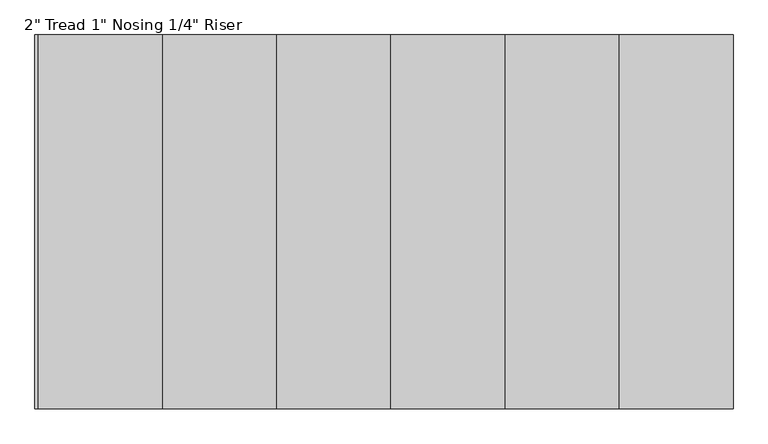
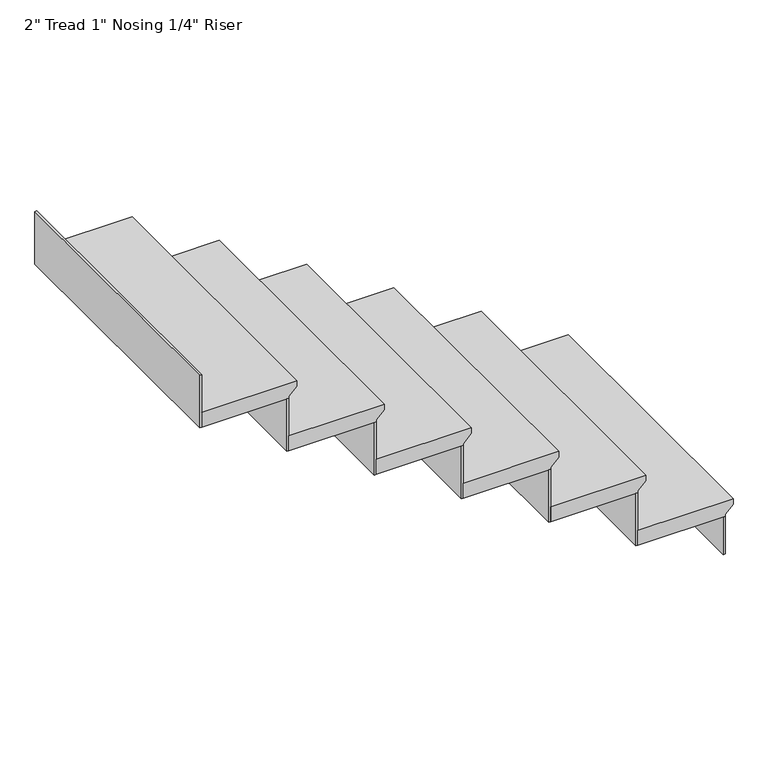
"""IFC4 building model written with IfcOpenShell, lengths in millimetres: stair flight geometry."""

from ifc_helpers import new_model, si_unit, origin, place, context, project, spatial, faceted_brep, source, transform, mapped, element, save


def stair_flight_17170d3d(model_context):
    return source(origin(), model_context, "Body", "Brep", [
        faceted_brep([(-6576.0763529, -1051.6338022, 768.35), (-6576.0763529, -1051.6338022, 787.4), (-6576.0763529, -1966.0338022, 787.4), (-6576.0763529, -1966.0338022, 768.35), (-6601.4763529, -1051.6338022, 742.95), (-6601.4763529, -1966.0338022, 742.95), (-6880.8763529, -1051.6338022, 787.4), (-6880.8763529, -1966.0338022, 787.4), (-6601.4763529, -1966.0338022, 736.6), (-6880.8763529, -1966.0338022, 736.6), (-6880.8763529, -1051.6338022, 736.6), (-6601.4763529, -1051.6338022, 736.6)], [[[0, 1, 2, 3]], [[4, 0, 3, 5]], [[2, 1, 6, 7]], [[8, 9, 10, 11]], [[2, 7, 9, 8, 5, 3]], [[8, 11, 4, 5]], [[6, 1, 0, 4, 11, 10]], [[7, 6, 10, 9]]]),
        faceted_brep([(-6601.4763529, -1051.6338022, 736.6), (-6601.4763529, -1051.6338022, 609.6), (-6607.8263529, -1051.6338022, 609.6), (-6607.8263529, -1051.6338022, 736.6), (-6601.4763529, -1966.0338022, 736.6), (-6607.8263529, -1966.0338022, 736.6), (-6607.8263529, -1966.0338022, 609.6), (-6601.4763529, -1966.0338022, 609.6)], [[[0, 1, 2, 3]], [[4, 5, 6, 7]], [[1, 0, 4, 7]], [[2, 1, 7, 6]], [[3, 2, 6, 5]], [[0, 3, 5, 4]]]),
        faceted_brep([(-6880.8763529, -1051.6338022, 914.4), (-6880.8763529, -1051.6338022, 736.6), (-6887.2263529, -1051.6338022, 736.6), (-6887.2263529, -1051.6338022, 914.4), (-6880.8763529, -1966.0338022, 914.4), (-6887.2263529, -1966.0338022, 914.4), (-6887.2263529, -1966.0338022, 736.6), (-6880.8763529, -1966.0338022, 736.6)], [[[0, 1, 2, 3]], [[4, 5, 6, 7]], [[1, 0, 4, 7]], [[2, 1, 7, 6]], [[3, 2, 6, 5]], [[0, 3, 5, 4]]]),
        faceted_brep([(-6855.4763529, -1966.0338022, 965.2), (-6855.4763529, -1051.6338022, 965.2), (-7160.2763529, -1051.6338022, 965.2), (-7160.2763529, -1966.0338022, 965.2), (-6880.8763529, -1966.0338022, 914.4), (-7160.2763529, -1966.0338022, 914.4), (-7160.2763529, -1051.6338022, 914.4), (-6880.8763529, -1051.6338022, 914.4), (-6880.8763529, -1966.0338022, 920.75), (-6855.4763529, -1966.0338022, 946.15), (-6880.8763529, -1051.6338022, 920.75), (-6855.4763529, -1051.6338022, 946.15)], [[[0, 1, 2, 3]], [[4, 5, 6, 7]], [[0, 3, 5, 4, 8, 9]], [[4, 7, 10, 8]], [[2, 1, 11, 10, 7, 6]], [[3, 2, 6, 5]], [[11, 1, 0, 9]], [[10, 11, 9, 8]]]),
        faceted_brep([(-7160.2763529, -1051.6338022, 1092.2), (-7160.2763529, -1051.6338022, 914.4), (-7166.6263529, -1051.6338022, 914.4), (-7166.6263529, -1051.6338022, 1092.2), (-7160.2763529, -1966.0338022, 1092.2), (-7166.6263529, -1966.0338022, 1092.2), (-7166.6263529, -1966.0338022, 914.4), (-7160.2763529, -1966.0338022, 914.4)], [[[0, 1, 2, 3]], [[4, 5, 6, 7]], [[1, 0, 4, 7]], [[2, 1, 7, 6]], [[3, 2, 6, 5]], [[0, 3, 5, 4]]]),
        faceted_brep([(-7134.8763529, -1966.0338022, 1143.0), (-7134.8763529, -1051.6338022, 1143.0), (-7439.6763529, -1051.6338022, 1143.0), (-7439.6763529, -1966.0338022, 1143.0), (-7160.2763529, -1966.0338022, 1092.2), (-7439.6763529, -1966.0338022, 1092.2), (-7439.6763529, -1051.6338022, 1092.2), (-7160.2763529, -1051.6338022, 1092.2), (-7160.2763529, -1966.0338022, 1098.55), (-7134.8763529, -1966.0338022, 1123.95), (-7160.2763529, -1051.6338022, 1098.55), (-7134.8763529, -1051.6338022, 1123.95)], [[[0, 1, 2, 3]], [[4, 5, 6, 7]], [[0, 3, 5, 4, 8, 9]], [[4, 7, 10, 8]], [[2, 1, 11, 10, 7, 6]], [[3, 2, 6, 5]], [[11, 1, 0, 9]], [[10, 11, 9, 8]]]),
        faceted_brep([(-7439.6763529, -1051.6338022, 1270.0), (-7439.6763529, -1051.6338022, 1092.2), (-7446.0263529, -1051.6338022, 1092.2), (-7446.0263529, -1051.6338022, 1270.0), (-7439.6763529, -1966.0338022, 1270.0), (-7446.0263529, -1966.0338022, 1270.0), (-7446.0263529, -1966.0338022, 1092.2), (-7439.6763529, -1966.0338022, 1092.2)], [[[0, 1, 2, 3]], [[4, 5, 6, 7]], [[1, 0, 4, 7]], [[2, 1, 7, 6]], [[3, 2, 6, 5]], [[0, 3, 5, 4]]]),
        faceted_brep([(-7414.2763529, -1966.0338022, 1320.8), (-7414.2763529, -1051.6338022, 1320.8), (-7719.0763529, -1051.6338022, 1320.8), (-7719.0763529, -1966.0338022, 1320.8), (-7439.6763529, -1966.0338022, 1270.0), (-7719.0763529, -1966.0338022, 1270.0), (-7719.0763529, -1051.6338022, 1270.0), (-7439.6763529, -1051.6338022, 1270.0), (-7439.6763529, -1966.0338022, 1276.35), (-7414.2763529, -1966.0338022, 1301.75), (-7439.6763529, -1051.6338022, 1276.35), (-7414.2763529, -1051.6338022, 1301.75)], [[[0, 1, 2, 3]], [[4, 5, 6, 7]], [[0, 3, 5, 4, 8, 9]], [[4, 7, 10, 8]], [[2, 1, 11, 10, 7, 6]], [[3, 2, 6, 5]], [[11, 1, 0, 9]], [[10, 11, 9, 8]]]),
        faceted_brep([(-7719.0763529, -1051.6338022, 1447.8), (-7719.0763529, -1051.6338022, 1270.0), (-7725.4263529, -1051.6338022, 1270.0), (-7725.4263529, -1051.6338022, 1447.8), (-7719.0763529, -1966.0338022, 1447.8), (-7725.4263529, -1966.0338022, 1447.8), (-7725.4263529, -1966.0338022, 1270.0), (-7719.0763529, -1966.0338022, 1270.0)], [[[0, 1, 2, 3]], [[4, 5, 6, 7]], [[1, 0, 4, 7]], [[2, 1, 7, 6]], [[3, 2, 6, 5]], [[0, 3, 5, 4]]]),
        faceted_brep([(-7693.6763529, -1966.0338022, 1498.6), (-7693.6763529, -1051.6338022, 1498.6), (-7998.4763529, -1051.6338022, 1498.6), (-7998.4763529, -1966.0338022, 1498.6), (-7719.0763529, -1966.0338022, 1447.8), (-7998.4763529, -1966.0338022, 1447.8), (-7998.4763529, -1051.6338022, 1447.8), (-7719.0763529, -1051.6338022, 1447.8), (-7719.0763529, -1966.0338022, 1454.15), (-7693.6763529, -1966.0338022, 1479.55), (-7719.0763529, -1051.6338022, 1454.15), (-7693.6763529, -1051.6338022, 1479.55)], [[[0, 1, 2, 3]], [[4, 5, 6, 7]], [[0, 3, 5, 4, 8, 9]], [[4, 7, 10, 8]], [[2, 1, 11, 10, 7, 6]], [[3, 2, 6, 5]], [[11, 1, 0, 9]], [[10, 11, 9, 8]]]),
        faceted_brep([(-8277.8763529, -1051.6338022, 1803.4), (-8277.8763529, -1051.6338022, 1625.6), (-8284.2263529, -1051.6338022, 1625.6), (-8284.2263529, -1051.6338022, 1803.4), (-8277.8763529, -1966.0338022, 1803.4), (-8284.2263529, -1966.0338022, 1803.4), (-8284.2263529, -1966.0338022, 1625.6), (-8277.8763529, -1966.0338022, 1625.6)], [[[0, 1, 2, 3]], [[4, 5, 6, 7]], [[1, 0, 4, 7]], [[2, 1, 7, 6]], [[3, 2, 6, 5]], [[0, 3, 5, 4]]]),
        faceted_brep([(-7998.4763529, -1051.6338022, 1625.6), (-7998.4763529, -1051.6338022, 1447.8), (-8004.8263529, -1051.6338022, 1447.8), (-8004.8263529, -1051.6338022, 1625.6), (-7998.4763529, -1966.0338022, 1625.6), (-8004.8263529, -1966.0338022, 1625.6), (-8004.8263529, -1966.0338022, 1447.8), (-7998.4763529, -1966.0338022, 1447.8)], [[[0, 1, 2, 3]], [[4, 5, 6, 7]], [[1, 0, 4, 7]], [[2, 1, 7, 6]], [[3, 2, 6, 5]], [[0, 3, 5, 4]]]),
        faceted_brep([(-7973.0763529, -1966.0338022, 1676.4), (-7973.0763529, -1051.6338022, 1676.4), (-8252.4763529, -1051.6338022, 1676.4), (-8277.8763529, -1051.6338022, 1676.4), (-8277.8763529, -1966.0338022, 1676.4), (-7998.4763529, -1966.0338022, 1625.6), (-8277.8763529, -1966.0338022, 1625.6), (-8277.8763529, -1051.6338022, 1625.6), (-8252.4763529, -1051.6338022, 1625.6), (-7998.4763529, -1051.6338022, 1625.6), (-7998.4763529, -1966.0338022, 1631.95), (-7973.0763529, -1966.0338022, 1657.35), (-7998.4763529, -1051.6338022, 1631.95), (-7973.0763529, -1051.6338022, 1657.35)], [[[0, 1, 2, 3, 4]], [[5, 6, 7, 8, 9]], [[0, 4, 6, 5, 10, 11]], [[5, 9, 12, 10]], [[2, 1, 13, 12, 9, 8]], [[3, 2, 8, 7]], [[4, 3, 7, 6]], [[13, 1, 0, 11]], [[12, 13, 11, 10]]]),
    ])


if __name__ == "__main__":
    model = new_model("IFC4")
    model_context = context("Model", 3, world=origin())
    ifc_project = project(units=[si_unit("LENGTHUNIT", "METRE", prefix="MILLI")], contexts=[model_context])
    site = spatial("IfcSite", under=ifc_project)
    building = spatial("IfcBuilding", under=site)
    placement = place(None, origin())
    stair_flight_shape = stair_flight_17170d3d(model_context)
    element("IfcStairFlight", 1, ObjectType="2\" Tread 1\" Nosing 1/4\" Riser", at=placement, inside=building, context=model_context, shape_type="MappedRepresentation", body=[
        mapped(stair_flight_shape, transform((0.0, 0.0, 0.0), x_axis=(1.0, 0.0, 0.0), y_axis=(0.0, 1.0, 0.0), z_axis=(0.0, 0.0, 1.0))),
    ])
    save(model, "model.ifc")
